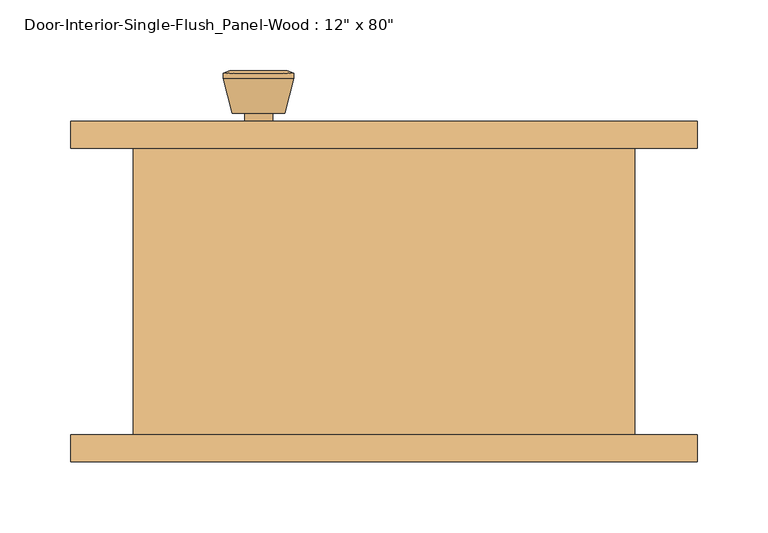
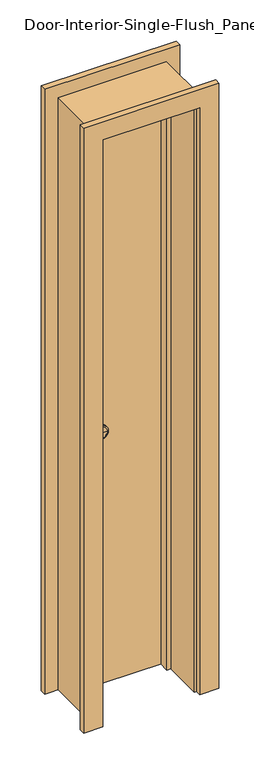
"""IFC4 building model written with IfcOpenShell, lengths in millimetres: door geometry."""

from ifc_helpers import new_model, si_unit, point, frame, frame_2d, origin, origin_with_axes, place, context, project, spatial, polyline, circle_curve, trimmed, segment, composite_curve, outline, extrude, faceted_brep, source, transform, mapped, element, save
from ifc_brep_helpers import plane_surface, cylinder_surface, revolved_surface, advanced_brep


def door_b2d2822a(model_context):
    return source(origin(), model_context, "Body", "SolidModel", [
        advanced_brep(
        [(-88.9, 57.5, 914.4), (-78.9, 57.5, 914.4), (-98.9, 57.5, 914.4), (-68.4241324, 8.5, 914.4), (-88.9, 8.5, 914.4), (-109.3758676, 8.5, 914.4), (-63.9, 10.3278681, 914.4), (-113.9, 10.3278681, 914.4), (-63.9, 13.7915463, 914.4), (-113.9, 13.7915463, 914.4), (-70.263764, 38.5, 914.4), (-107.536236, 38.5, 914.4), (-78.9, 38.5, 914.4), (-98.9, 38.5, 914.4)],
        [
            (0, 1),
            (1, 2, circle_curve(frame((-88.9, 57.5, 914.4), z_axis=(0.0, 1.0, 0.0), x_axis=(-1.0, 0.0, 0.0)), 10.0)),
            (2, 0),
            (2, 1, circle_curve(frame((-88.9, 57.5, 914.4), z_axis=(0.0, 1.0, 0.0), x_axis=(-1.0, 0.0, 0.0)), 10.0)),
            (3, 4),
            (4, 5),
            (5, 3, circle_curve(frame((-88.9, 8.5, 914.4), z_axis=(0.0, -1.0, 0.0), x_axis=(-1.0, 0.0, 0.0)), 20.4758676)),
            (3, 5, circle_curve(frame((-88.9, 8.5, 914.4), z_axis=(0.0, -1.0, 0.0), x_axis=(-1.0, 0.0, 0.0)), 20.4758676)),
            (6, 3),
            (5, 7),
            (7, 6, circle_curve(frame((-88.9, 10.3278681, 914.4), z_axis=(0.0, -1.0, 0.0), x_axis=(-1.0, 0.0, 0.0)), 25.0)),
            (6, 7, circle_curve(frame((-88.9, 10.3278681, 914.4), z_axis=(0.0, -1.0, 0.0), x_axis=(-1.0, 0.0, 0.0)), 25.0)),
            (8, 6),
            (7, 9),
            (9, 8, circle_curve(frame((-88.9, 13.7915463, 914.4), z_axis=(0.0, -1.0, 0.0), x_axis=(-1.0, 0.0, 0.0)), 25.0)),
            (8, 9, circle_curve(frame((-88.9, 13.7915463, 914.4), z_axis=(0.0, -1.0, 0.0), x_axis=(-1.0, 0.0, 0.0)), 25.0)),
            (10, 8),
            (9, 11),
            (11, 10, circle_curve(frame((-88.9, 38.5, 914.4), z_axis=(0.0, -1.0, 0.0), x_axis=(-1.0, 0.0, 0.0)), 18.636236)),
            (10, 11, circle_curve(frame((-88.9, 38.5, 914.4), z_axis=(0.0, -1.0, 0.0), x_axis=(-1.0, 0.0, 0.0)), 18.636236)),
            (12, 10),
            (11, 13),
            (13, 12, circle_curve(frame((-88.9, 38.5, 914.4), z_axis=(0.0, -1.0, 0.0), x_axis=(-1.0, 0.0, 0.0)), 10.0)),
            (12, 13, circle_curve(frame((-88.9, 38.5, 914.4), z_axis=(0.0, -1.0, 0.0), x_axis=(-1.0, 0.0, 0.0)), 10.0)),
            (1, 12),
            (13, 2),
        ],
        [
            plane_surface(frame((-88.9, 57.5, 914.4), z_axis=(0.0, 1.0, 0.0), x_axis=(-1.0, 0.0, 0.0))),
            plane_surface(frame((-88.9, 8.5, 914.4), z_axis=(0.0, -1.0, 0.0), x_axis=(-1.0, 0.0, 0.0))),
            revolved_surface(polyline([(-109.3758676, 8.5, 914.4), (-113.9, 10.3278681, 914.4)]), (-88.9, 57.5, 914.4), (0.0, 1.0, 0.0)),
            cylinder_surface(frame((-88.9, 57.5, 914.4), z_axis=(0.0, 1.0, 0.0), x_axis=(-1.0, 0.0, 0.0)), 25.0),
            revolved_surface(polyline([(-113.9, 13.7915463, 914.4), (-107.536236, 38.5, 914.4)]), (-88.9, 57.5, 914.4), (0.0, 1.0, 0.0)),
            plane_surface(frame((-88.9, 38.5, 914.4), z_axis=(0.0, 1.0, 0.0), x_axis=(-1.0, 0.0, 0.0))),
            cylinder_surface(frame((-88.9, 57.5, 914.4), z_axis=(0.0, 1.0, 0.0), x_axis=(-1.0, 0.0, 0.0)), 10.0),
        ],
        [
            (0, [[1, 2, 3]]),
            (0, [[-3, 4, -1]]),
            (1, [[5, 6, 7]]),
            (1, [[-6, -5, 8]]),
            (2, [[9, -7, 10, 11]]),
            (2, [[-10, -8, -9, 12]]),
            (3, [[13, -11, 14, 15]]),
            (3, [[-14, -12, -13, 16]]),
            (4, [[17, -15, 18, 19]]),
            (4, [[-18, -16, -17, 20]]),
            (5, [[21, -19, 22, 23]]),
            (5, [[-22, -20, -21, 24]]),
            (6, [[25, -23, 26, -2]]),
            (6, [[-26, -24, -25, -4]]),
        ],
    ),
        extrude(outline(composite_curve([segment(trimmed(circle_curve(frame_2d((914.4, -88.9)), 30.0), [point((914.4, -118.9))], [point((914.4, -58.9))], False, "CARTESIAN"), True, "CONTINUOUS"), segment(trimmed(circle_curve(frame_2d((914.4, -88.9)), 30.0), [point((914.4, -58.9))], [point((914.4, -118.9))], False, "CARTESIAN"), True, "CONTINUOUS")], self_intersect=False)), frame((0.0, 57.5, 0.0), z_axis=(0.0, 1.0, 0.0), x_axis=(0.0, 0.0, 1.0)), (0.0, 0.0, 1.0), 6.0),
        advanced_brep(
        [(-88.9, 104.425, 914.4), (-98.9, 104.425, 914.4), (-78.9, 104.425, 914.4), (-68.4241324, 153.425, 914.4), (-109.3758676, 153.425, 914.4), (-88.9, 153.425, 914.4), (-63.9, 151.5971319, 914.4), (-113.9, 151.5971319, 914.4), (-63.9, 148.1334537, 914.4), (-113.9, 148.1334537, 914.4), (-70.263764, 123.425, 914.4), (-107.536236, 123.425, 914.4), (-78.9, 123.425, 914.4), (-98.9, 123.425, 914.4)],
        [
            (0, 1),
            (1, 2, circle_curve(frame((-88.9, 104.425, 914.4), z_axis=(0.0, -1.0, 0.0), x_axis=(-1.0, 0.0, 0.0)), 10.0)),
            (2, 0),
            (2, 1, circle_curve(frame((-88.9, 104.425, 914.4), z_axis=(0.0, -1.0, 0.0), x_axis=(-1.0, 0.0, 0.0)), 10.0)),
            (3, 4, circle_curve(frame((-88.9, 153.425, 914.4), z_axis=(0.0, 1.0, 0.0), x_axis=(-1.0, 0.0, 0.0)), 20.4758676)),
            (4, 5),
            (5, 3),
            (4, 3, circle_curve(frame((-88.9, 153.425, 914.4), z_axis=(0.0, 1.0, 0.0), x_axis=(-1.0, 0.0, 0.0)), 20.4758676)),
            (6, 7, circle_curve(frame((-88.9, 151.5971319, 914.4), z_axis=(0.0, 1.0, 0.0), x_axis=(-1.0, 0.0, 0.0)), 25.0)),
            (7, 4),
            (3, 6),
            (7, 6, circle_curve(frame((-88.9, 151.5971319, 914.4), z_axis=(0.0, 1.0, 0.0), x_axis=(-1.0, 0.0, 0.0)), 25.0)),
            (8, 9, circle_curve(frame((-88.9, 148.1334537, 914.4), z_axis=(0.0, 1.0, 0.0), x_axis=(-1.0, 0.0, 0.0)), 25.0)),
            (9, 7),
            (6, 8),
            (9, 8, circle_curve(frame((-88.9, 148.1334537, 914.4), z_axis=(0.0, 1.0, 0.0), x_axis=(-1.0, 0.0, 0.0)), 25.0)),
            (10, 11, circle_curve(frame((-88.9, 123.425, 914.4), z_axis=(0.0, 1.0, 0.0), x_axis=(-1.0, 0.0, 0.0)), 18.636236)),
            (11, 9),
            (8, 10),
            (11, 10, circle_curve(frame((-88.9, 123.425, 914.4), z_axis=(0.0, 1.0, 0.0), x_axis=(-1.0, 0.0, 0.0)), 18.636236)),
            (12, 13, circle_curve(frame((-88.9, 123.425, 914.4), z_axis=(0.0, 1.0, 0.0), x_axis=(-1.0, 0.0, 0.0)), 10.0)),
            (13, 11),
            (10, 12),
            (13, 12, circle_curve(frame((-88.9, 123.425, 914.4), z_axis=(0.0, 1.0, 0.0), x_axis=(-1.0, 0.0, 0.0)), 10.0)),
            (1, 13),
            (12, 2),
        ],
        [
            plane_surface(frame((-88.9, 104.425, 914.4), z_axis=(0.0, -1.0, 0.0), x_axis=(-1.0, 0.0, 0.0))),
            plane_surface(frame((-88.9, 153.425, 914.4), z_axis=(0.0, 1.0, 0.0), x_axis=(-1.0, 0.0, 0.0))),
            revolved_surface(polyline([(-109.3758676, 153.425, 914.4), (-113.9, 151.5971319, 914.4)]), (-88.9, 104.425, 914.4), (0.0, -1.0, 0.0)),
            cylinder_surface(frame((-88.9, 104.425, 914.4), z_axis=(0.0, -1.0, 0.0), x_axis=(-1.0, 0.0, 0.0)), 25.0),
            revolved_surface(polyline([(-113.9, 148.1334537, 914.4), (-107.536236, 123.425, 914.4)]), (-88.9, 104.425, 914.4), (0.0, -1.0, 0.0)),
            plane_surface(frame((-88.9, 123.425, 914.4), z_axis=(0.0, -1.0, 0.0), x_axis=(-1.0, 0.0, 0.0))),
            cylinder_surface(frame((-88.9, 104.425, 914.4), z_axis=(0.0, -1.0, 0.0), x_axis=(-1.0, 0.0, 0.0)), 10.0),
        ],
        [
            (0, [[1, 2, 3]]),
            (0, [[-3, 4, -1]]),
            (1, [[5, 6, 7]]),
            (1, [[8, -7, -6]]),
            (2, [[9, 10, -5, 11]]),
            (2, [[12, -11, -8, -10]]),
            (3, [[13, 14, -9, 15]]),
            (3, [[16, -15, -12, -14]]),
            (4, [[17, 18, -13, 19]]),
            (4, [[20, -19, -16, -18]]),
            (5, [[21, 22, -17, 23]]),
            (5, [[24, -23, -20, -22]]),
            (6, [[-2, 25, -21, 26]]),
            (6, [[-4, -26, -24, -25]]),
        ],
    ),
        extrude(outline(composite_curve([segment(trimmed(circle_curve(frame_2d((914.4, -88.9)), 30.0), [point((914.4, -118.9))], [point((914.4, -58.9))], False, "CARTESIAN"), True, "CONTINUOUS"), segment(trimmed(circle_curve(frame_2d((914.4, -88.9)), 30.0), [point((914.4, -58.9))], [point((914.4, -118.9))], False, "CARTESIAN"), True, "CONTINUOUS")], self_intersect=False)), frame((0.0, 98.425, 0.0), z_axis=(0.0, 1.0, 0.0), x_axis=(0.0, 0.0, 1.0)), (0.0, 0.0, 1.0), 6.0),
        extrude(outline(polyline([(152.4, 63.5), (-152.4, 63.5), (-152.4, 98.425), (152.4, 98.425), (152.4, 63.5)])), origin_with_axes(), (0.0, 0.0, 1.0), 2032.0),
        faceted_brep([(177.8, 98.425, 0.0), (177.8, -104.775, 0.0), (152.4, -104.775, 0.0), (152.4, 28.575, 0.0), (139.7, 28.575, 0.0), (139.7, 63.5, 0.0), (152.4, 63.5, 0.0), (152.4, 98.425, 0.0), (177.8, 98.425, 2057.4), (177.8, -104.775, 2057.4), (-177.8, -104.775, 2057.4), (-177.8, -104.775, 0.0), (-152.4, -104.775, 0.0), (-152.4, -104.775, 2032.0), (152.4, -104.775, 2032.0), (152.4, 28.575, 2032.0), (-152.4, 28.575, 2032.0), (-152.4, 28.575, 0.0), (-139.7, 28.575, 0.0), (-139.7, 28.575, 2019.3), (139.7, 28.575, 2019.3), (139.7, 63.5, 2019.3), (-139.7, 63.5, 2019.3), (-139.7, 63.5, 0.0), (-152.4, 63.5, 0.0), (-152.4, 63.5, 2032.0), (152.4, 63.5, 2032.0), (152.4, 98.425, 2032.0), (-152.4, 98.425, 2032.0), (-152.4, 98.425, 0.0), (-177.8, 98.425, 0.0), (-177.8, 98.425, 2057.4)], [[[0, 1, 2, 3, 4, 5, 6, 7]], [[1, 0, 8, 9]], [[2, 1, 9, 10, 11, 12, 13, 14]], [[3, 2, 14, 15]], [[4, 3, 15, 16, 17, 18, 19, 20]], [[5, 4, 20, 21]], [[6, 5, 21, 22, 23, 24, 25, 26]], [[7, 6, 26, 27]], [[0, 7, 27, 28, 29, 30, 31, 8]], [[9, 8, 31, 10]], [[15, 14, 13, 16]], [[21, 20, 19, 22]], [[27, 26, 25, 28]], [[30, 29, 24, 23, 18, 17, 12, 11]], [[10, 31, 30, 11]], [[16, 13, 12, 17]], [[22, 19, 18, 23]], [[28, 25, 24, 29]]]),
        extrude(outline(polyline([(0.0, 158.75), (0.0, 222.25), (2101.85, 222.25), (2101.85, -222.25), (0.0, -222.25), (0.0, -158.75), (2038.35, -158.75), (2038.35, 158.75), (0.0, 158.75)])), frame((0.0, -123.825, 0.0), z_axis=(0.0, 1.0, 0.0), x_axis=(0.0, 0.0, 1.0)), (0.0, 0.0, 1.0), 19.05),
        extrude(outline(polyline([(0.0, 158.75), (0.0, 222.25), (2101.85, 222.25), (2101.85, -222.25), (0.0, -222.25), (0.0, -158.75), (2038.35, -158.75), (2038.35, 158.75), (0.0, 158.75)])), frame((0.0, 98.425, 0.0), z_axis=(0.0, 1.0, 0.0), x_axis=(0.0, 0.0, 1.0)), (0.0, 0.0, 1.0), 19.05),
    ])


if __name__ == "__main__":
    model = new_model("IFC4")
    model_context = context("Model", 3, world=origin())
    ifc_project = project(units=[si_unit("LENGTHUNIT", "METRE", prefix="MILLI")], contexts=[model_context])
    site = spatial("IfcSite", under=ifc_project)
    building = spatial("IfcBuilding", under=site)
    placement = place(None, origin())
    door_shape = door_b2d2822a(model_context)
    element("IfcDoor", 1, ObjectType="Door-Interior-Single-Flush_Panel-Wood : 12\" x 80\"", at=placement, inside=building, context=model_context, shape_type="MappedRepresentation", body=[
        mapped(door_shape, transform((0.0, 0.0, 0.0), x_axis=(1.0, 0.0, 0.0), y_axis=(0.0, 1.0, 0.0), z_axis=(0.0, 0.0, 1.0))),
    ])
    save(model, "model.ifc")

# Revit data of these elements
# Type "Door-Interior-Single-Flush_Panel-Wood : 12\" x 80\""
#   Type Mark = "9"
#   Assembly Code = "C1020300"
#   Analytic Construction = "Wooden"
#   Thickness = 0' - 1 3/8"
#   Thermal Resistance (R) = 2.5876 (h·ft²·°F)/BTU
#   Swing Angle [instance default] = 90.00°
#   Rough Width = 1' - 2"
#   Rough Height = 6' - 9"
#   Height = 6' - 8"
#   Width = 1' - 0"
#   Heat Transfer Coefficient (U) = 0.3865 BTU/(h·ft²·°F)
#   Trim Material = Cherry
#   Panel Material = Cherry
#   Frame Material = Cherry
#   Door Handle Material = Aluminum
#   Visual Light Transmittance = 0
#   Solar Heat Gain Coefficient = 0
#   Wall Closure = (empty or 0)
#   Function = (empty or 0)
# Element 1 (IfcDoor, "Door-Interior-Single-Flush_Panel-Wood : 12\" x 80\"")
#   Materials on its faces: "Cherry", "Aluminum"
# Materials
#   "Cherry": class "Wood", colour RGB 226 177 128, transparency 0, Description = "Prunus Serotina", Cost = 0
#   "Aluminum": class "Metal", colour RGB 247 247 247, transparency 0, Description = "Aluminum 6061", Cost = 0
